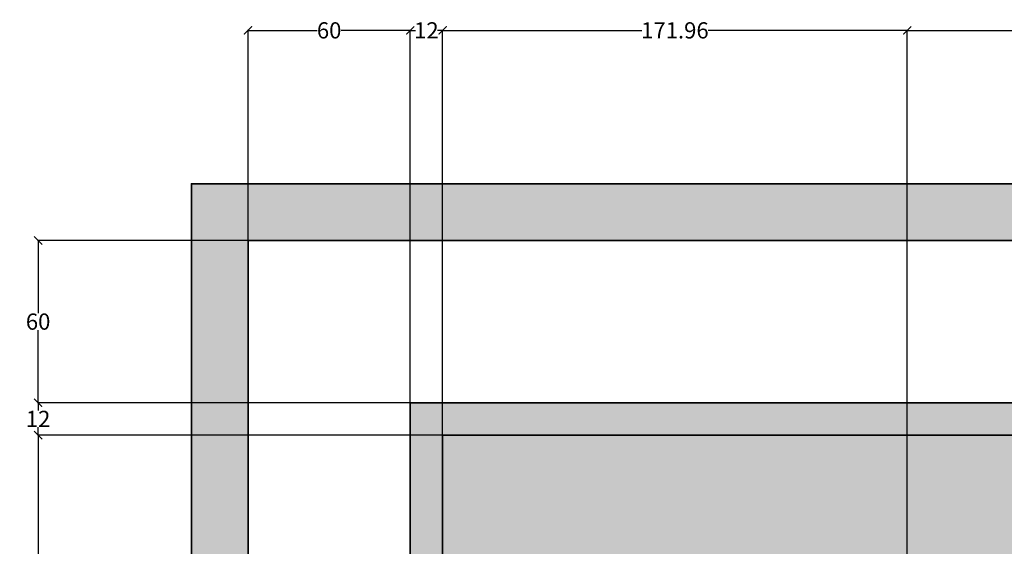
# Model space of a CAD drawing. Units: inches. Extents: x 925 to 2834, y 111 to 1355.
# Tile 16 of 25: x 928 to 1293, y 1160 to 1355. Entities that reach past the tile are written whole.
import ezdxf

# ---------------------------------------------------------------- set-up
doc = ezdxf.new("R2010")
doc.units = ezdxf.units.IN
doc.header["$MEASUREMENT"] = 0
for name, color, linetype, lineweight in [('A-ANNO-DIMS', 2, 'Continuous', 18), ('A-ANNO-TTLB', 7, 'Continuous', 35), ('A-FLOR-PATT', 252, 'Continuous', 13)]:
    doc.layers.add(name, color=color, linetype=linetype, lineweight=lineweight)
doc.styles.get("Standard").update_dxf_attribs({"font": 'arial.ttf'})
doc.dimstyles.get("Standard").update_dxf_attribs({"dimtxt": 6, "dimasz": 3, "dimexe": 0.18, "dimexo": 0.0625, "dimgap": 0.09, "dimtad": 0, "dimtih": 1, "dimtoh": 1, "dimdec": 1, "dimzin": 0, "dimdsep": 46, "dimlunit": 3, "dimtxsty": 'Standard', "dimblk": 'ARCHTICK', "dimcen": 0.09, "dimadec": 0, "dimazin": 0, "dimtfac": 1, "dimtdec": 1, "dimtofl": 0, "dimtmove": 0, "dimatfit": 3, "dimfxl": 1, "dimtolj": 1, "dimtzin": 0, "dimarcsym": 0})

# ---------------------------------------------------------------- blocks, each defined once
blk = doc.blocks.new('_ArchTick')
at = {"color": 0, "linetype": 'ByBlock', "const_width": 0.15}
blk.add_lwpolyline([(-0.5, -0.5), (0.5, 0.5)], dxfattribs=at)
blk = doc.blocks.new('*D13')
at = {"layer": 'A-ANNO-DIMS', "color": 0, "lineweight": -2, "transparency": 16777216}
for p, q in [((1012.71, 1273.65), (1012.71, 1351.49)), ((1012.71, 1351.31), (1038.32, 1351.31)), ((1072.71, 1351.31), (1047.11, 1351.31)), ((1072.71, 1213.65), (1072.71, 1351.49))]:
    blk.add_line(p, q, dxfattribs=at)
at = {"layer": 'Defpoints', "color": 0, "transparency": 16777216}
for p in [(1072.71, 1351.31), (1012.71, 1273.59), (1072.71, 1213.59)]:
    blk.add_point(p, dxfattribs=at)
at = {"layer": 'A-ANNO-DIMS', "color": 0, "lineweight": -2, "transparency": 16777216, "xscale": 3, "yscale": 3, "zscale": 3, "rotation": 180}
blk.add_blockref('_ArchTick', (1012.71, 1351.31), dxfattribs=at)
at = {"layer": 'A-ANNO-DIMS', "color": 0, "lineweight": -2, "transparency": 16777216, "xscale": 3, "yscale": 3, "zscale": 3}
blk.add_blockref('_ArchTick', (1072.71, 1351.31), dxfattribs=at)
at = {"layer": 'A-ANNO-DIMS', "color": 0, "transparency": 16777216, "insert": (1042.71, 1351.31), "char_height": 6, "attachment_point": 5}
blk.add_mtext('\\A1;60', dxfattribs=at)
blk = doc.blocks.new('*D14')
at = {"layer": 'A-ANNO-DIMS', "color": 0, "lineweight": -2, "transparency": 16777216}
for p, q in [((1072.71, 1213.65), (1072.71, 1351.49)), ((1072.71, 1351.31), (1074.64, 1351.31)), ((1084.71, 1351.31), (1082.79, 1351.31)), ((1084.71, 1201.65), (1084.71, 1351.49))]:
    blk.add_line(p, q, dxfattribs=at)
at = {"layer": 'Defpoints', "color": 0, "transparency": 16777216}
for p in [(1084.71, 1351.31), (1072.71, 1213.59), (1084.71, 1201.59)]:
    blk.add_point(p, dxfattribs=at)
at = {"layer": 'A-ANNO-DIMS', "color": 0, "lineweight": -2, "transparency": 16777216, "xscale": 3, "yscale": 3, "zscale": 3, "rotation": 180}
blk.add_blockref('_ArchTick', (1072.71, 1351.31), dxfattribs=at)
at = {"layer": 'A-ANNO-DIMS', "color": 0, "lineweight": -2, "transparency": 16777216, "xscale": 3, "yscale": 3, "zscale": 3}
blk.add_blockref('_ArchTick', (1084.71, 1351.31), dxfattribs=at)
at = {"layer": 'A-ANNO-DIMS', "color": 0, "transparency": 16777216, "insert": (1078.71, 1351.31), "char_height": 6, "attachment_point": 5}
blk.add_mtext('\\A1;12', dxfattribs=at)
blk = doc.blocks.new('*D15')
at = {"layer": 'A-ANNO-DIMS', "color": 0, "lineweight": -2, "transparency": 16777216}
for p, q in [((1084.71, 1081.65), (1084.71, 1351.49)), ((1084.71, 1351.31), (1158.43, 1351.31)), ((1256.67, 1351.31), (1182.95, 1351.31)), ((1256.67, 1081.65), (1256.67, 1351.49))]:
    blk.add_line(p, q, dxfattribs=at)
at = {"layer": 'Defpoints', "color": 0, "transparency": 16777216}
for p in [(1256.67, 1351.31), (1084.71, 1081.59), (1256.67, 1081.59)]:
    blk.add_point(p, dxfattribs=at)
at = {"layer": 'A-ANNO-DIMS', "color": 0, "lineweight": -2, "transparency": 16777216, "xscale": 3, "yscale": 3, "zscale": 3, "rotation": 180}
blk.add_blockref('_ArchTick', (1084.71, 1351.31), dxfattribs=at)
at = {"layer": 'A-ANNO-DIMS', "color": 0, "lineweight": -2, "transparency": 16777216, "xscale": 3, "yscale": 3, "zscale": 3}
blk.add_blockref('_ArchTick', (1256.67, 1351.31), dxfattribs=at)
at = {"layer": 'A-ANNO-DIMS', "color": 0, "transparency": 16777216, "insert": (1170.69, 1351.31), "char_height": 6, "attachment_point": 5}
blk.add_mtext('\\A1;171.96', dxfattribs=at)
blk = doc.blocks.new('*D16')
at = {"layer": 'A-ANNO-DIMS', "color": 0, "lineweight": -2, "transparency": 16777216}
for p, q in [((1256.67, 1081.65), (1256.67, 1351.49)), ((1256.67, 1351.31), (1412.16, 1351.31)), ((1592.71, 1351.31), (1437.22, 1351.31)), ((1592.71, 1071.65), (1592.71, 1351.49))]:
    blk.add_line(p, q, dxfattribs=at)
at = {"layer": 'Defpoints', "color": 0, "transparency": 16777216}
for p in [(1592.71, 1351.31), (1256.67, 1081.59), (1592.71, 1071.59)]:
    blk.add_point(p, dxfattribs=at)
at = {"layer": 'A-ANNO-DIMS', "color": 0, "lineweight": -2, "transparency": 16777216, "xscale": 3, "yscale": 3, "zscale": 3, "rotation": 180}
blk.add_blockref('_ArchTick', (1256.67, 1351.31), dxfattribs=at)
at = {"layer": 'A-ANNO-DIMS', "color": 0, "lineweight": -2, "transparency": 16777216, "xscale": 3, "yscale": 3, "zscale": 3}
blk.add_blockref('_ArchTick', (1592.71, 1351.31), dxfattribs=at)
at = {"layer": 'A-ANNO-DIMS', "color": 0, "transparency": 16777216, "insert": (1424.69, 1351.31), "char_height": 6, "attachment_point": 5}
blk.add_mtext('\\A1;336.04', dxfattribs=at)
blk = doc.blocks.new('*D37')
at = {"layer": 'A-ANNO-DIMS', "color": 0, "lineweight": -2, "transparency": 16777216}
for p, q in [((1084.65, 1201.59), (934.81, 1201.59)), ((934.99, 1201.59), (934.99, 1144.74)), ((934.99, 1081.59), (934.99, 1138.44)), ((1084.65, 1081.59), (934.81, 1081.59))]:
    blk.add_line(p, q, dxfattribs=at)
at = {"layer": 'Defpoints', "color": 0, "transparency": 16777216}
for p in [(934.99, 1201.59), (1084.71, 1201.59), (1084.71, 1081.59)]:
    blk.add_point(p, dxfattribs=at)
at = {"layer": 'A-ANNO-DIMS', "color": 0, "lineweight": -2, "transparency": 16777216, "xscale": 3, "yscale": 3, "zscale": 3}
for p, rotation in [((934.99, 1201.59), 90), ((934.99, 1081.59), 270)]:
    blk.add_blockref('_ArchTick', p, dxfattribs=dict(at, rotation=rotation))
at = {"layer": 'A-ANNO-DIMS', "color": 0, "transparency": 16777216, "insert": (934.99, 1141.59), "char_height": 6, "attachment_point": 5}
blk.add_mtext('\\A1;120', dxfattribs=at)
blk = doc.blocks.new('*D38')
at = {"layer": 'A-ANNO-DIMS', "color": 0, "lineweight": -2, "transparency": 16777216}
for p, q in [((1072.65, 1213.59), (934.81, 1213.59)), ((934.99, 1213.59), (934.99, 1210.69)), ((934.99, 1201.59), (934.99, 1204.49)), ((1084.65, 1201.59), (934.81, 1201.59))]:
    blk.add_line(p, q, dxfattribs=at)
at = {"layer": 'Defpoints', "color": 0, "transparency": 16777216}
for p in [(934.99, 1213.59), (1072.71, 1213.59), (1084.71, 1201.59)]:
    blk.add_point(p, dxfattribs=at)
at = {"layer": 'A-ANNO-DIMS', "color": 0, "lineweight": -2, "transparency": 16777216, "xscale": 3, "yscale": 3, "zscale": 3}
for p, rotation in [((934.99, 1213.59), 90), ((934.99, 1201.59), 270)]:
    blk.add_blockref('_ArchTick', p, dxfattribs=dict(at, rotation=rotation))
at = {"layer": 'A-ANNO-DIMS', "color": 0, "transparency": 16777216, "insert": (934.99, 1207.59), "char_height": 6, "attachment_point": 5}
blk.add_mtext('\\A1;12', dxfattribs=at)
blk = doc.blocks.new('*D39')
at = {"layer": 'A-ANNO-DIMS', "color": 0, "lineweight": -2, "transparency": 16777216}
for p, q in [((1012.65, 1273.59), (934.81, 1273.59)), ((934.99, 1273.59), (934.99, 1246.74)), ((934.99, 1213.59), (934.99, 1240.44)), ((1072.65, 1213.59), (934.81, 1213.59))]:
    blk.add_line(p, q, dxfattribs=at)
at = {"layer": 'Defpoints', "color": 0, "transparency": 16777216}
for p in [(934.99, 1273.59), (1012.71, 1273.59), (1072.71, 1213.59)]:
    blk.add_point(p, dxfattribs=at)
at = {"layer": 'A-ANNO-DIMS', "color": 0, "lineweight": -2, "transparency": 16777216, "xscale": 3, "yscale": 3, "zscale": 3}
for p, rotation in [((934.99, 1273.59), 90), ((934.99, 1213.59), 270)]:
    blk.add_blockref('_ArchTick', p, dxfattribs=dict(at, rotation=rotation))
at = {"layer": 'A-ANNO-DIMS', "color": 0, "transparency": 16777216, "insert": (934.99, 1243.59), "char_height": 6, "attachment_point": 5}
blk.add_mtext('\\A1;60', dxfattribs=at)

msp = doc.modelspace()

# ---------------------------------------------------------------- hatches: boundary and pattern name
at = {"layer": 'A-FLOR-PATT', "transparency": 33554605}
h = msp.add_hatch(color=256, dxfattribs=at)
h.dxf.hatch_style = 1
h.paths.add_polyline_path([(1931.688, 1294.5638), (991.7375, 1294.5638), (991.7375, 172.1134), (1931.688, 172.1134)])
h.paths.add_polyline_path([(1910.7128, 1273.5886), (1910.7128, 193.0886), (1012.7128, 193.0886), (1012.7128, 1273.5886)], flags=16)
h.paths.add_polyline_path([(1850.7128, 1213.5886), (1850.7128, 253.0886), (1072.7128, 253.0886), (1072.7128, 1213.5886)], flags=0)
h.paths.add_polyline_path([(1838.7128, 1201.5886), (1838.7128, 265.0886), (1084.7128, 265.0886), (1084.7128, 530.5886), (1084.7128, 1201.5886)], flags=0)
h.paths.add_polyline_path([(1547.6758, 1155.7396), (1547.6758, 1119.115), (1513.0687, 1119.115), (1513.0687, 1155.7396)], flags=0)
h.paths.add_polyline_path([(1600.1067, 1154.9439), (1634.7139, 1154.9439), (1634.7139, 1119.115), (1600.1067, 1119.115)], flags=0)
h.paths.add_polyline_path([(1505.2502, 1144.5358), (1505.2502, 1119.115), (1470.643, 1119.115), (1470.643, 1144.5358)], flags=0)
h.paths.add_polyline_path([(1559.1357, 1141.0962), (1593.7428, 1141.0962), (1593.7428, 1119.115), (1559.1357, 1119.115)], flags=0)
h.paths.add_polyline_path([(1462.8966, 1154.9439), (1462.8966, 1119.115), (1428.2895, 1119.115), (1428.2895, 1154.9439)], flags=0)
h.paths.add_polyline_path([(1642.4603, 1144.5358), (1677.0675, 1144.5358), (1677.0675, 1119.115), (1642.4603, 1119.115)], flags=0)
h.paths.add_polyline_path([(1422.3508, 1141.0962), (1422.3508, 1119.115), (1387.7436, 1119.115), (1387.7436, 1141.0962)], flags=0)
h.paths.add_polyline_path([(1684.8859, 1155.7396), (1719.4931, 1155.7396), (1719.4931, 1119.115), (1684.8859, 1119.115)], flags=0)
h.paths.add_polyline_path([(1718.7128, 1081.5886), (1718.7128, 1050.1249), (1715.7128, 1050.1249), (1715.7128, 1026.1249), (1715.7128, 1002.1249), (1718.7128, 1002.1249), (1730.7128, 1002.1249), (1730.7128, 998.1249), (1730.7128, 990.1249), (1730.7128, 986.1249), (1718.7128, 986.1249), (1718.7128, 893.5886), (1715.3735, 893.5886), (1715.3735, 891.5886), (1713.3735, 891.5886, 0.41421356), (1677.3735, 855.5886), (1713.3735, 855.5886), (1713.3735, 853.5886), (1715.3735, 853.5886), (1715.3735, 851.5886), (1718.7128, 851.5886), (1718.7128, 821.5865), (1734.4655, 821.5865), (1734.3735, 819.5886, -0.41421356), (1712.4415, 793.5886), (1712.4415, 791.5886), (1718.7128, 791.5886), (1718.7128, 717.5886), (1718.7128, 669.5886), (1732.7128, 669.5886), (1732.7128, 665.5886), (1732.7128, 641.5886), (1732.7128, 634.5886), (1732.7128, 610.5886), (1732.7128, 603.5886), (1718.7128, 603.5886), (1718.7128, 385.0886), (1434.2128, 385.0886), (1434.2128, 530.5886), (1410.2128, 530.5886), (1408.2128, 530.5886), (1408.2128, 532.5886, 0.41421356), (1372.2128, 568.5886), (1372.2128, 532.5886), (1370.2128, 532.5886), (1370.2128, 530.5886), (1368.2128, 530.5886), (1282.2128, 530.5886), (1210.2128, 530.5886), (1200.2128, 530.5886), (1200.2128, 542.1915), (1183.2307, 542.1915), (1183.2307, 546.1915), (1200.2128, 546.1915), (1200.2128, 572.1915), (1183.2307, 572.1915), (1183.2307, 576.1915), (1200.2128, 576.1915), (1200.2128, 727.5886), (1210.2128, 727.5886), (1234.2128, 727.5886), (1259.7128, 727.5886), (1259.7128, 775.5886), (1259.7128, 799.5886), (1259.7128, 847.5886), (1259.7128, 993.5872), (1259.7128, 1065.5872), (1259.7128, 1071.5886), (1219.6318, 1071.5886), (1219.6318, 1081.5886), (1084.7128, 1081.5886), (1084.7128, 1119.115), (1256.8974, 1119.115), (1256.8974, 1154.9439), (1291.5046, 1154.9439), (1291.5046, 1119.115), (1256.8974, 1119.115), (1256.6723, 1081.5886), (1293.7128, 1081.5886), (1341.7128, 1081.5886), (1341.7128, 1093.5886), (1347.7128, 1093.5886), (1371.7128, 1093.5886), (1377.7128, 1093.5886), (1377.7128, 1081.5886), (1668.7128, 1081.5886), (1668.7128, 1117.5886), (1675.7128, 1117.5886), (1711.7128, 1117.5886), (1718.7128, 1117.5886)], flags=0)
h.paths.add_polyline_path([(1376.2838, 1155.7396), (1376.2838, 1119.115), (1341.6766, 1119.115), (1341.6766, 1155.7396)], flags=0)
h.paths.add_polyline_path([(1341.7128, 1076.0886), (1293.7128, 1076.0886), (1293.7128, 1071.5886), (1269.7128, 1071.5886), (1269.7128, 1065.5872), (1266.7128, 1065.5872), (1266.7128, 1029.5872), (1265.7128, 1029.5872), (1265.7128, 993.5872), (1269.7128, 993.5872), (1269.7128, 903.5886), (1269.7128, 893.5886), (1269.7128, 847.5886), (1265.2128, 847.5886), (1265.2128, 799.5886), (1269.7128, 799.5886), (1269.7128, 775.5886), (1265.2128, 775.5886), (1265.2128, 727.5886), (1269.7128, 727.5886), (1444.2128, 727.5886), (1444.2128, 717.5886), (1234.2128, 717.5886), (1234.2128, 722.0886), (1210.2128, 722.0886), (1210.2128, 717.5886), (1210.2128, 540.5886), (1210.2128, 536.0886), (1282.2128, 536.0886), (1282.2128, 535.0886), (1210.2128, 535.0886), (1210.2128, 540.5886), (1210.2128, 717.5886), (1210.2128, 723.0886), (1234.2128, 723.0886), (1234.2128, 717.5886), (1444.2128, 717.5886), (1444.2128, 727.5886), (1269.7128, 727.5886), (1264.2128, 727.5886), (1264.2128, 775.5886), (1269.7128, 775.5886), (1269.7128, 799.5886), (1264.2128, 799.5886), (1264.2128, 847.5886), (1269.7128, 847.5886), (1269.7128, 893.5886), (1269.7128, 903.5886), (1269.7128, 993.5872), (1264.7128, 993.5872), (1264.7128, 1029.5872), (1265.7128, 1029.5872), (1265.7128, 1065.5872), (1269.7128, 1065.5872), (1269.7128, 1071.5886), (1293.7128, 1071.5886), (1293.7128, 1077.0886), (1341.7128, 1077.0886)], flags=0)
h.paths.add_polyline_path([(1730.9529, 1141.0962), (1765.5601, 1141.0962), (1765.5601, 1119.115), (1730.9529, 1119.115)], flags=0)
h.paths.add_polyline_path([(1333.8582, 1144.5358), (1333.8582, 1119.115), (1299.251, 1119.115), (1299.251, 1144.5358)], flags=0)
h.paths.add_polyline_path([(1592.7128, 968.5886), (1596.0342, 968.5886), (1602.7128, 968.5886), (1708.7128, 968.5886), (1708.7128, 903.5886), (1602.7128, 903.5886), (1602.7128, 938.5886), (1592.7128, 938.5886), (1592.7128, 903.5886), (1451.7128, 903.5886), (1451.7128, 893.5886), (1511.7128, 893.5886), (1511.7128, 881.5886), (1515.2128, 881.5886), (1518.7128, 881.5886), (1518.7128, 893.5886), (1592.7128, 893.5886), (1592.7128, 799.5886), (1518.7128, 799.5886), (1518.7128, 857.5886), (1511.7128, 857.5886), (1511.7128, 799.5886), (1511.7128, 772.0886), (1521.7128, 772.0886), (1521.7128, 792.5886), (1592.7128, 792.5886), (1592.7128, 727.5886), (1521.7128, 727.5886), (1521.7128, 748.0886), (1511.7128, 748.0886), (1511.7128, 717.5886), (1708.7128, 717.5886), (1714.2128, 717.5886), (1714.2128, 669.5886), (1708.7128, 669.5886), (1708.7128, 641.5886), (1492.2128, 641.5886), (1492.2128, 631.5886), (1621.2128, 631.5886), (1621.2128, 443.0886), (1625.7128, 443.0886), (1625.7128, 503.0886), (1625.7128, 507.5886), (1625.7128, 631.5886), (1708.7128, 631.5886), (1708.7128, 507.5886), (1655.7128, 507.5886), (1655.7128, 503.0886), (1708.7128, 503.0886), (1708.7128, 395.0886), (1625.7128, 395.0886), (1625.7128, 419.0886), (1621.2128, 419.0886), (1621.2128, 395.0886), (1482.2128, 395.0886), (1482.2128, 385.0886), (1434.2128, 385.0886), (1434.2128, 433.0886), (1444.2128, 433.0886), (1444.2128, 631.5886), (1450.2128, 631.5886), (1450.2128, 634.91), (1452.2128, 634.91), (1452.2128, 669.5886), (1454.2128, 669.5886, -0.40021217), (1490.1712, 635.3173), (1492.2128, 635.3173), (1492.2128, 641.5886), (1564.7128, 641.5886), (1564.7128, 677.5886), (1672.7128, 677.5886), (1672.7128, 681.5886), (1564.7128, 681.5886), (1564.7128, 717.5886), (1511.7128, 717.5886), (1511.7128, 748.0886), (1511.7128, 772.0886), (1511.7128, 799.5886), (1511.7128, 857.5886), (1511.8913, 857.5886), (1511.8913, 859.5886), (1515.6201, 859.5886, 0.41421356), (1537.552, 879.5886), (1513.552, 879.5886), (1511.8913, 879.5886), (1511.8913, 881.5886), (1511.7128, 881.5886), (1511.7128, 893.5886), (1451.7128, 893.5886), (1451.7128, 903.5886), (1592.7128, 903.5886), (1592.7128, 938.5886), (1592.7128, 940.5886), (1596.4415, 940.5886, 0.41421356), (1618.3735, 966.5886), (1594.3735, 966.5886), (1592.7128, 966.5886)], flags=0)
h.paths.add_polyline_path([(1377.7128, 903.5886), (1377.7128, 893.5886), (1305.7128, 893.5886), (1305.7128, 903.5886)], flags=0)
h.paths.add_polyline_path([(1708.7128, 821.5886), (1712.0342, 821.5886), (1712.0342, 819.5886), (1710.3735, 819.5886), (1708.7128, 819.5886)], flags=0)
h.paths.add_polyline_path([(1576.7128, 695.1992), (1575.5896, 693.6649), (1575.9687, 694.6994), (1575.4438, 695.1992), (1575.9687, 695.699), (1575.5896, 696.7335)], flags=0)
h.paths.add_polyline_path([(1565.9817, 662.3134), (1565.4568, 661.8136), (1565.8359, 660.7791), (1564.7128, 662.3134), (1565.8359, 663.8477), (1565.4568, 662.8132)], flags=0)
h.paths.add_polyline_path([(1444.2128, 433.0886), (1444.2128, 395.0886), (1482.2128, 395.0886), (1482.2128, 389.0886), (1438.2128, 389.0886), (1438.2128, 391.8608), (1438.2128, 433.0886)], flags=0)
h.paths.add_polyline_path([(1410.2128, 506.5886), (1410.2128, 289.0886), (1108.7128, 289.0886), (1108.7128, 506.5886)], flags=0)
h.paths.add_polyline_path([(1612.3153, 838.3016), (1680.4151, 838.3016), (1680.4151, 851.3131), (1612.3153, 851.3131)], flags=8)
h.paths.add_polyline_path([(1208.3174, 395.0436), (1282.1017, 395.0436), (1282.1017, 408.0552), (1208.3174, 408.0552)], flags=8)
h.paths.add_polyline_path([(1291.8049, 598.7427), (1369.8017, 598.7427), (1369.8017, 611.7542), (1291.8049, 611.7542)], flags=8)
h.paths.add_polyline_path([(1119.679, 917.3022), (1191.0817, 917.3022), (1191.0817, 930.3137), (1119.679, 930.3137)], flags=8)
h.paths.add_polyline_path([(1332.2261, 815.9808), (1410.2258, 815.9808), (1410.2258, 829.001), (1332.2261, 829.001)], flags=8)
h.paths.add_polyline_path([(1390.9013, 955.8158), (1475.4981, 955.8158), (1475.4981, 968.8273), (1390.9013, 968.8273)], flags=8)
h.paths.add_polyline_path([(1620.3436, 998.9325), (1688.4434, 998.9325), (1688.4434, 1011.944), (1620.3436, 1011.944)], flags=8)
h.paths.add_polyline_path([(1620.3436, 914.1039), (1691.7405, 914.1039), (1691.7405, 927.1155), (1620.3436, 927.1155)], flags=8)
h.paths.add_polyline_path([(1521.4542, 816.005), (1589.5569, 816.005), (1589.5569, 829.0253), (1521.4542, 829.0253)], flags=8)
h.paths.add_polyline_path([(1528.524, 740.3497), (1602.3082, 740.3497), (1602.3082, 753.3613), (1528.524, 753.3613)], flags=8)
h.paths.add_polyline_path([(1627.6094, 762.6128), (1702.3091, 762.6128), (1702.3091, 775.6244), (1627.6094, 775.6244)], flags=8)
h.paths.add_polyline_path([(1610.5442, 657.2751), (1684.3284, 657.2751), (1684.3284, 670.2867), (1610.5442, 670.2867)], flags=8)
h.paths.add_polyline_path([(1636.6983, 519.472), (1711.3981, 519.472), (1711.3981, 532.4835), (1636.6983, 532.4835)], flags=8)
h.paths.add_polyline_path([(1616.8577, 424.8539), (1694.8545, 424.8539), (1694.8545, 437.8654), (1616.8577, 437.8654)], flags=8)
h.paths.add_polyline_path([(1506.1456, 460.8838), (1579.9299, 460.8838), (1579.9299, 473.8953), (1506.1456, 473.8953)], flags=8)
h.paths.add_polyline_path([(1624.6119, 784.6011), (1696.9185, 784.6011), (1696.9185, 797.7864), (1624.6119, 797.7864)], flags=8)
h.paths.add_polyline_path([(1606.3732, 854.2194), (1683.3039, 854.2194), (1683.3039, 867.4048), (1606.3732, 867.4048)], flags=8)
h.paths.add_polyline_path([(1127.8008, 940.3581), (1165.1637, 940.3581), (1165.1637, 953.5348), (1127.8008, 953.5348)], flags=8)
h.paths.add_polyline_path([(1620.8657, 1019.4968), (1677.3447, 1019.4968), (1677.3447, 1032.6735), (1620.8657, 1032.6735)], flags=8)
h.paths.add_polyline_path([(1620.8643, 930.1821), (1703.0564, 930.1821), (1703.0564, 943.3675), (1620.8643, 943.3675)], flags=8)
h.paths.add_polyline_path([(1324.5702, 836.8338), (1408.0892, 836.8338), (1408.0892, 850.0191), (1324.5702, 850.0191)], flags=8)
h.paths.add_polyline_path([(1281.6584, 622.8885), (1383.6213, 622.8885), (1383.6213, 636.0739), (1281.6584, 636.0739)], flags=8)
h.paths.add_polyline_path([(1210.6721, 416.7893), (1269.1299, 416.7893), (1269.1299, 429.9747), (1210.6721, 429.9747)], flags=8)
h.paths.add_polyline_path([(1507.8264, 477.4836), (1586.7329, 477.4836), (1586.7329, 490.669), (1507.8264, 490.669)], flags=8)
h.paths.add_polyline_path([(1643.6238, 443.8135), (1696.6696, 443.8135), (1696.6696, 456.5643), (1643.6238, 456.5643)], flags=8)
h.paths.add_polyline_path([(1647.2466, 540.5638), (1693.1825, 540.5638), (1693.1825, 553.7491), (1647.2466, 553.7491)], flags=8)
h.paths.add_polyline_path([(1626.0633, 668.5064), (1673.3174, 668.5064), (1673.3174, 681.6831), (1626.0633, 681.6831)], flags=8)
h.paths.add_polyline_path([(1538.2915, 830.7872), (1567.5942, 830.7872), (1567.5942, 843.5293), (1538.2915, 843.5293)], flags=8)
h.paths.add_polyline_path([(1530.9338, 754.0477), (1559.576, 754.0477), (1559.576, 766.7898), (1530.9338, 766.7898)], flags=8)
h.paths.add_polyline_path([(1351.2461, 979.2309), (1513.8919, 979.2309), (1513.8919, 992.4076), (1351.2461, 992.4076)], flags=8)
at = {"layer": 'A-FLOR-PATT'}
h = msp.add_hatch(color=256, dxfattribs=at)
h.dxf.hatch_style = 1
h.paths.add_polyline_path([(1850.7128, 1213.5886), (1072.7128, 1213.5886), (1072.7128, 253.0886), (1850.7128, 253.0886)])
h.paths.add_polyline_path([(1084.7128, 1201.5886), (1838.7128, 1201.5886), (1838.7128, 265.0886), (1084.7128, 265.0886)], flags=16)
h.paths.add_polyline_path([(1183.2307, 576.1915), (1200.2128, 576.1915), (1200.2128, 727.5886), (1210.2128, 727.5886), (1234.2128, 727.5886), (1259.7128, 727.5886), (1259.7128, 775.5886), (1259.7128, 799.5886), (1259.7128, 847.5886), (1259.7128, 993.5872), (1259.7128, 1065.5872), (1259.7128, 1071.5886), (1219.6318, 1071.5886), (1219.6318, 1081.5886), (1293.7128, 1081.5886), (1341.7128, 1081.5886), (1341.7128, 1093.5886), (1347.7128, 1093.5886), (1347.7128, 1081.5886), (1371.7128, 1081.5886), (1371.7128, 1093.5886), (1377.7128, 1093.5886), (1377.7128, 1081.5886), (1668.7128, 1081.5886), (1668.7128, 1117.5886), (1675.7128, 1117.5886), (1675.7128, 1081.5886), (1711.7128, 1081.5886), (1711.7128, 1117.5886), (1718.7128, 1117.5886), (1718.7128, 1081.5886), (1718.7128, 1050.1249), (1715.7128, 1050.1249), (1715.7128, 1026.1249), (1715.7128, 1002.1249), (1718.7128, 1002.1249), (1730.7128, 1002.1249), (1730.7128, 998.1249), (1730.7128, 990.1249), (1730.7128, 986.1249), (1718.7128, 986.1249), (1718.7128, 893.5886), (1715.3735, 893.5886), (1715.3735, 891.5886), (1713.3735, 891.5886, 0.41421356), (1677.3735, 855.5886), (1713.3735, 855.5886), (1713.3735, 853.5886), (1715.3735, 853.5886), (1715.3735, 851.5886), (1718.7128, 851.5886), (1718.7128, 821.5865), (1734.4655, 821.5865), (1734.3735, 819.5886, -0.41421356), (1712.4415, 793.5886), (1712.4415, 791.5886), (1718.7128, 791.5886), (1718.7128, 717.5886), (1718.7128, 669.5886), (1732.7128, 669.5886), (1732.7128, 665.5886), (1732.7128, 641.5886), (1732.7128, 634.5886), (1732.7128, 610.5886), (1732.7128, 603.5886), (1718.7128, 603.5886), (1718.7128, 385.0886), (1434.2128, 385.0886), (1434.2128, 433.0886), (1434.2128, 530.5886), (1410.2128, 530.5886), (1408.2128, 530.5886), (1408.2128, 532.5886, 0.41421356), (1372.2128, 568.5886), (1372.2128, 532.5886), (1370.2128, 532.5886), (1370.2128, 530.5886), (1368.2128, 530.5886), (1282.2128, 530.5886), (1210.2128, 530.5886), (1200.2128, 530.5886), (1200.2128, 542.1915), (1183.2307, 542.1915), (1183.2307, 546.1915), (1200.2128, 546.1915), (1200.2128, 572.1915), (1183.2307, 572.1915)], flags=0)
h.paths.add_polyline_path([(1210.2128, 717.5886), (1210.2128, 723.0886), (1234.2128, 723.0886), (1234.2128, 717.5886), (1444.2128, 717.5886), (1444.2128, 727.5886), (1269.7128, 727.5886), (1264.2128, 727.5886), (1264.2128, 775.5886), (1269.7128, 775.5886), (1269.7128, 799.5886), (1264.2128, 799.5886), (1264.2128, 847.5886), (1269.7128, 847.5886), (1269.7128, 893.5886), (1269.7128, 903.5886), (1269.7128, 993.5872), (1264.7128, 993.5872), (1264.7128, 1029.5872), (1265.7128, 1029.5872), (1265.7128, 1065.5872), (1269.7128, 1065.5872), (1269.7128, 1071.5886), (1293.7128, 1071.5886), (1293.7128, 1077.0886), (1341.7128, 1077.0886), (1341.7128, 1076.0886), (1293.7128, 1076.0886), (1293.7128, 1071.5886), (1269.7128, 1071.5886), (1269.7128, 1065.5872), (1266.7128, 1065.5872), (1266.7128, 1029.5872), (1265.7128, 1029.5872), (1265.7128, 993.5872), (1269.7128, 993.5872), (1269.7128, 903.5886), (1269.7128, 893.5886), (1269.7128, 847.5886), (1265.2128, 847.5886), (1265.2128, 799.5886), (1269.7128, 799.5886), (1269.7128, 775.5886), (1265.2128, 775.5886), (1265.2128, 727.5886), (1269.7128, 727.5886), (1444.2128, 727.5886), (1444.2128, 717.5886), (1234.2128, 717.5886), (1234.2128, 722.0886), (1210.2128, 722.0886), (1210.2128, 717.5886), (1210.2128, 540.5886), (1210.2128, 536.0886), (1282.2128, 536.0886), (1282.2128, 535.0886), (1210.2128, 535.0886), (1210.2128, 540.5886)], flags=0)
h.paths.add_polyline_path([(1450.2128, 634.91), (1452.2128, 634.91), (1452.2128, 669.5886), (1454.2128, 669.5886, -0.40021217), (1490.1712, 635.3173), (1492.2128, 635.3173), (1492.2128, 641.5886), (1564.7128, 641.5886), (1564.7128, 677.5886), (1672.7128, 677.5886), (1672.7128, 681.5886), (1564.7128, 681.5886), (1564.7128, 717.5886), (1511.7128, 717.5886), (1511.7128, 748.0886), (1511.7128, 772.0886), (1511.7128, 799.5886), (1511.7128, 857.5886), (1511.8913, 857.5886), (1511.8913, 859.5886), (1515.6201, 859.5886, 0.41421356), (1537.552, 879.5886), (1513.552, 879.5886), (1511.8913, 879.5886), (1511.8913, 881.5886), (1511.7128, 881.5886), (1511.7128, 893.5886), (1451.7128, 893.5886), (1451.7128, 903.5886), (1592.7128, 903.5886), (1592.7128, 938.5886), (1592.7128, 940.5886), (1596.4415, 940.5886, 0.41421356), (1618.3735, 966.5886), (1594.3735, 966.5886), (1592.7128, 966.5886), (1592.7128, 968.5886), (1596.0342, 968.5886), (1602.7128, 968.5886), (1708.7128, 968.5886), (1708.7128, 903.5886), (1602.7128, 903.5886), (1602.7128, 938.5886), (1592.7128, 938.5886), (1592.7128, 903.5886), (1451.7128, 903.5886), (1451.7128, 893.5886), (1511.7128, 893.5886), (1511.7128, 881.5886), (1518.7128, 881.5886), (1518.7128, 893.5886), (1592.7128, 893.5886), (1592.7128, 799.5886), (1518.7128, 799.5886), (1518.7128, 857.5886), (1511.7128, 857.5886), (1511.7128, 799.5886), (1511.7128, 772.0886), (1521.7128, 772.0886), (1521.7128, 792.5886), (1592.7128, 792.5886), (1592.7128, 727.5886), (1521.7128, 727.5886), (1521.7128, 748.0886), (1511.7128, 748.0886), (1511.7128, 717.5886), (1708.7128, 717.5886), (1714.2128, 717.5886), (1714.2128, 669.5886), (1708.7128, 669.5886), (1708.7128, 641.5886), (1492.2128, 641.5886), (1492.2128, 631.5886), (1621.2128, 631.5886), (1621.2128, 443.0886), (1625.7128, 443.0886), (1625.7128, 503.0886), (1625.7128, 507.5886), (1625.7128, 631.5886), (1708.7128, 631.5886), (1708.7128, 507.5886), (1655.7128, 507.5886), (1655.7128, 503.0886), (1708.7128, 503.0886), (1708.7128, 395.0886), (1625.7128, 395.0886), (1625.7128, 419.0886), (1621.2128, 419.0886), (1621.2128, 395.0886), (1482.2128, 395.0886), (1482.2128, 389.0886), (1438.2128, 389.0886), (1438.2128, 391.8608), (1438.2128, 433.0886), (1444.2128, 433.0886), (1444.2128, 631.5886), (1450.2128, 631.5886)], flags=0)
h.paths.add_polyline_path([(1444.2128, 433.0886), (1444.2128, 395.0886), (1482.2128, 395.0886), (1482.2128, 391.0886), (1440.2128, 391.0886), (1440.2128, 391.8608), (1440.2128, 433.0886)], flags=0)
h.paths.add_polyline_path([(1305.7128, 893.5886), (1305.7128, 903.5886), (1377.7128, 903.5886), (1377.7128, 893.5886)], flags=0)
h.paths.add_polyline_path([(1564.7128, 662.3134), (1565.8359, 663.8477), (1565.4568, 662.8132), (1565.9817, 662.3134), (1565.4568, 661.8136), (1565.8359, 660.7791)], flags=0)
h.paths.add_polyline_path([(1575.4438, 695.1992), (1575.9687, 695.699), (1575.5896, 696.7335), (1576.7128, 695.1992), (1575.5896, 693.6649), (1575.9687, 694.6994)], flags=0)
h.paths.add_polyline_path([(1708.7128, 821.5886), (1712.0342, 821.5886), (1712.0342, 819.5886), (1710.3735, 819.5886), (1708.7128, 819.5886)], flags=0)
at = {"layer": 'A-FLOR-PATT', "transparency": 33554554}
h = msp.add_hatch(color=256, dxfattribs=at)
h.dxf.hatch_style = 1
h.paths.add_polyline_path([(1838.7128, 1201.5886), (1084.7128, 1201.5886), (1084.7128, 1119.115), (1256.8974, 1119.115), (1256.8974, 1154.9439), (1291.5046, 1154.9439), (1291.5046, 1119.115), (1256.8974, 1119.115), (1256.6723, 1081.5886), (1293.7128, 1081.5886), (1341.7128, 1081.5886), (1341.7128, 1093.5886), (1347.7128, 1093.5886), (1371.7128, 1093.5886), (1377.7128, 1093.5886), (1377.7128, 1081.5886), (1668.7128, 1081.5886), (1668.7128, 1117.5886), (1675.7128, 1117.5886), (1711.7128, 1117.5886), (1718.7128, 1117.5886), (1718.7128, 1081.5886), (1838.7128, 1081.5886)])
h.paths.add_polyline_path([(1299.251, 1144.5358), (1333.8582, 1144.5358), (1333.8582, 1119.115), (1299.251, 1119.115)], flags=16)
h.paths.add_polyline_path([(1341.6766, 1155.7396), (1376.2838, 1155.7396), (1376.2838, 1119.115), (1341.6766, 1119.115)], flags=16)
h.paths.add_polyline_path([(1387.7436, 1141.0962), (1422.3508, 1141.0962), (1422.3508, 1119.115), (1387.7436, 1119.115)], flags=16)
h.paths.add_polyline_path([(1428.2895, 1154.9439), (1462.8966, 1154.9439), (1462.8966, 1119.115), (1428.2895, 1119.115)], flags=16)
h.paths.add_polyline_path([(1470.643, 1144.5358), (1505.2502, 1144.5358), (1505.2502, 1119.115), (1470.643, 1119.115)], flags=16)
h.paths.add_polyline_path([(1513.0687, 1155.7396), (1547.6758, 1155.7396), (1547.6758, 1119.115), (1513.0687, 1119.115)], flags=16)
h.paths.add_polyline_path([(1559.1357, 1141.0962), (1593.7428, 1141.0962), (1593.7428, 1119.115), (1559.1357, 1119.115)], flags=16)
h.paths.add_polyline_path([(1600.1067, 1154.9439), (1634.7139, 1154.9439), (1634.7139, 1119.115), (1600.1067, 1119.115)], flags=16)
h.paths.add_polyline_path([(1642.4603, 1144.5358), (1677.0675, 1144.5358), (1677.0675, 1119.115), (1642.4603, 1119.115)], flags=16)
h.paths.add_polyline_path([(1684.8859, 1155.7396), (1719.4931, 1155.7396), (1719.4931, 1119.115), (1684.8859, 1119.115)], flags=16)
h.paths.add_polyline_path([(1730.9529, 1141.0962), (1765.5601, 1141.0962), (1765.5601, 1119.115), (1730.9529, 1119.115)], flags=16)

# ---------------------------------------------------------------- linework, layer by layer
at = {"layer": 'A-ANNO-TTLB'}
for points in [[(991.7375, 172.1134), (1931.688, 172.1134), (1931.688, 1294.5638), (991.7375, 1294.5638)], [(1012.7128, 193.0886), (1910.7128, 193.0886), (1910.7128, 1273.5886), (1012.7128, 1273.5886)], [(1072.7128, 253.0886), (1850.7128, 253.0886), (1850.7128, 1213.5886), (1072.7128, 1213.5886)], [(1084.7128, 265.0886), (1838.7128, 265.0886), (1838.7128, 1201.5886), (1084.7128, 1201.5886)]]:
    msp.add_lwpolyline(points, close=True, dxfattribs=at)

# ---------------------------------------------------------------- dimensions: what is measured, and where the dimension line sits
at = {"layer": 'A-ANNO-DIMS'}
for base, p1, p2, override, picture, middle in [((1072.7128, 1351.3138), (1012.7128, 1273.5886), (1072.7128, 1213.5886), {"dimdec": 0, "dimlfac": 1, "dimrnd": 0, "dimzin": 0, "dimdsep": 46, "dimlunit": 2}, '*D13', (1042.7128, 1351.3138)), ((1084.7128, 1351.3138), (1072.7128, 1213.5886), (1084.7128, 1201.5886), {"dimdec": 0, "dimlfac": 1, "dimrnd": 0, "dimzin": 0, "dimdsep": 46, "dimlunit": 2}, '*D14', (1078.7128, 1351.3138)), ((1256.6723, 1351.3138), (1084.7128, 1081.5886), (1256.6723, 1081.5886), {"dimdec": 2, "dimlfac": 1, "dimrnd": 0, "dimzin": 0, "dimdsep": 46, "dimlunit": 2}, '*D15', (1170.6925, 1351.3138)), ((1592.7128, 1351.3138), (1256.6723, 1081.5886), (1592.7128, 1071.5886), {"dimdec": 2, "dimlfac": 1, "dimrnd": 0, "dimzin": 0, "dimdsep": 46, "dimlunit": 2}, '*D16', (1424.6925, 1351.3138))]:
    dim = msp.add_linear_dim(base=base, p1=p1, p2=p2, dimstyle='Standard', override=override, dxfattribs=at)
    dim.commit()
    dim.dimension.update_dxf_attribs({"geometry": picture, "text_midpoint": middle})
for base, p1, p2, picture, middle in [((934.9875, 1273.5886), (1072.7128, 1213.5886), (1012.7128, 1273.5886), '*D39', (934.9875, 1243.5886)), ((934.9875, 1213.5886), (1084.7128, 1201.5886), (1072.7128, 1213.5886), '*D38', (934.9875, 1207.5886)), ((934.9875, 1201.5886), (1084.7128, 1081.5886), (1084.7128, 1201.5886), '*D37', (934.9875, 1141.5886))]:
    dim = msp.add_linear_dim(base=base, p1=p1, p2=p2, angle=90, dimstyle='Standard', override={"dimdec": 0, "dimlfac": 1, "dimrnd": 0, "dimzin": 0, "dimdsep": 46, "dimlunit": 2}, dxfattribs=at)
    dim.commit()
    dim.dimension.update_dxf_attribs({"geometry": picture, "text_midpoint": middle})

doc.saveas('drawing.dxf')
